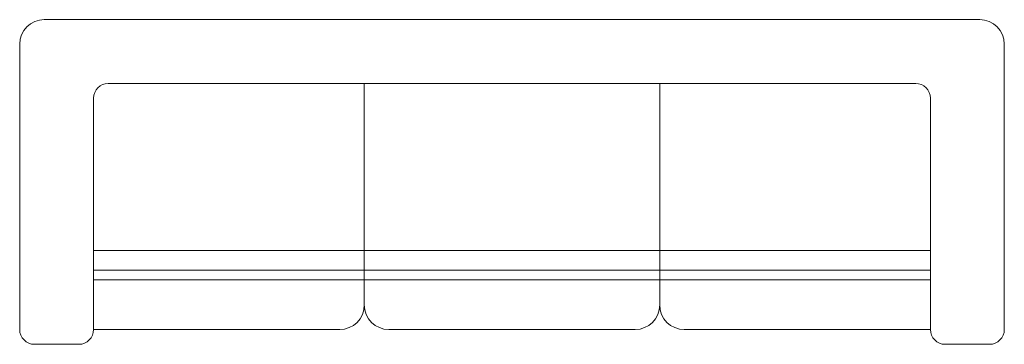
# Model space of a CAD drawing. Units: inches. Extents: x 2901 to 5923, y 918 to 2827.
# Tile 16 of 16: x 5923.0739 to 5923.15264, y 1249.35805 to 1249.38402. Entities that reach past the tile are written whole.
import ezdxf

# ---------------------------------------------------------------- set-up
doc = ezdxf.new("R2010")
doc.units = ezdxf.units.IN
doc.layers.add('furniture', color=160, linetype='Continuous', lineweight=18)

# ---------------------------------------------------------------- blocks, each defined once
blk = doc.blocks.new('A$C05BA3A2B')
for p, q in [((0.05, 0.6596), (1.95, 0.6596)), ((0.05, 0.6596), (1.95, 0.6596)), ((0.05, 0.6596), (1.95, 0.6596)), ((0, 0.03), (0, 0.6096)), ((0, 0.03), (0, 0.6096)), ((0, 0.03), (0, 0.6096)), ((2, 0.6096), (2, 0.03)), ((2, 0.6096), (2, 0.03)), ((2, 0.6096), (2, 0.03)), ((1.82, 0.53), (0.18, 0.53)), ((1.82, 0.53), (0.18, 0.53)), ((1.82, 0.53), (0.18, 0.53)), ((0.7, 0.08), (0.7, 0.53)), ((0.7, 0.08), (0.7, 0.53)), ((0.7, 0.08), (0.7, 0.53)), ((1.3, 0.53), (1.3, 0.08)), ((1.3, 0.53), (1.3, 0.08)), ((1.3, 0.53), (1.3, 0.08)), ((0.15, 0.5), (0.15, 0.03)), ((0.15, 0.5), (0.15, 0.03)), ((0.15, 0.5), (0.15, 0.03)), ((1.85, 0.03), (1.85, 0.5)), ((1.85, 0.03), (1.85, 0.5)), ((1.85, 0.03), (1.85, 0.5)), ((1.85, 0.1908), (0.15, 0.1908)), ((1.85, 0.1908), (0.15, 0.1908)), ((1.85, 0.1908), (0.15, 0.1908)), ((1.85, 0.1508), (0.15, 0.1508)), ((1.85, 0.1508), (0.15, 0.1508)), ((1.85, 0.1508), (0.15, 0.1508)), ((1.85, 0.1308), (0.15, 0.1308)), ((1.85, 0.1308), (0.15, 0.1308)), ((1.85, 0.1308), (0.15, 0.1308)), ((0.65, 0.03), (0.15, 0.03)), ((0.65, 0.03), (0.15, 0.03)), ((0.65, 0.03), (0.15, 0.03)), ((1.25, 0.03), (0.75, 0.03)), ((1.25, 0.03), (0.75, 0.03)), ((1.25, 0.03), (0.75, 0.03)), ((1.85, 0.03), (1.35, 0.03)), ((1.85, 0.03), (1.35, 0.03)), ((1.85, 0.03), (1.35, 0.03)), ((0.12, 0), (0.03, 0)), ((0.12, 0), (0.03, 0)), ((0.12, 0), (0.03, 0)), ((1.97, 0), (1.88, 0)), ((1.97, 0), (1.88, 0)), ((1.97, 0), (1.88, 0))]:
    blk.add_line(p, q)
for centre, radius, start, end in [((0.05, 0.6096), 0.05, 90, 180), ((0.05, 0.6096), 0.05, 90, 180), ((0.05, 0.6096), 0.05, 90, 180), ((1.95, 0.6096), 0.05, 0, 90), ((1.95, 0.6096), 0.05, 0, 90), ((1.95, 0.6096), 0.05, 0, 90), ((0.18, 0.5), 0.03, 90, 180), ((0.18, 0.5), 0.03, 90, 180), ((0.18, 0.5), 0.03, 90, 180), ((1.82, 0.5), 0.03, 0, 90), ((1.82, 0.5), 0.03, 0, 90), ((1.82, 0.5), 0.03, 0, 90), ((0.65, 0.08), 0.05, 270, 0), ((0.65, 0.08), 0.05, 270, 0), ((0.65, 0.08), 0.05, 270, 0), ((0.75, 0.08), 0.05, 180, 270), ((0.75, 0.08), 0.05, 180, 270), ((0.75, 0.08), 0.05, 180, 270), ((1.25, 0.08), 0.05, 270, 0), ((1.25, 0.08), 0.05, 270, 0), ((1.25, 0.08), 0.05, 270, 0), ((1.35, 0.08), 0.05, 180, 270), ((1.35, 0.08), 0.05, 180, 270), ((1.35, 0.08), 0.05, 180, 270), ((0.03, 0.03), 0.03, 180, 270), ((0.03, 0.03), 0.03, 180, 270), ((0.03, 0.03), 0.03, 180, 270), ((0.12, 0.03), 0.03, 270, 0), ((0.12, 0.03), 0.03, 270, 0), ((0.12, 0.03), 0.03, 270, 0), ((1.88, 0.03), 0.03, 180, 270), ((1.88, 0.03), 0.03, 180, 270), ((1.88, 0.03), 0.03, 180, 270), ((1.97, 0.03), 0.03, 270, 0), ((1.97, 0.03), 0.03, 270, 0), ((1.97, 0.03), 0.03, 270, 0)]:
    blk.add_arc(centre, radius, start, end)

msp = doc.modelspace()

# ---------------------------------------------------------------- block references
at = {"layer": 'furniture', "xscale": 0.0393700787401575, "yscale": 0.0393700787401575, "zscale": 0.0393700787401575}
msp.add_blockref('A$C05BA3A2B', (5923.073902, 1249.358051), dxfattribs=at)

doc.saveas('drawing.dxf')
